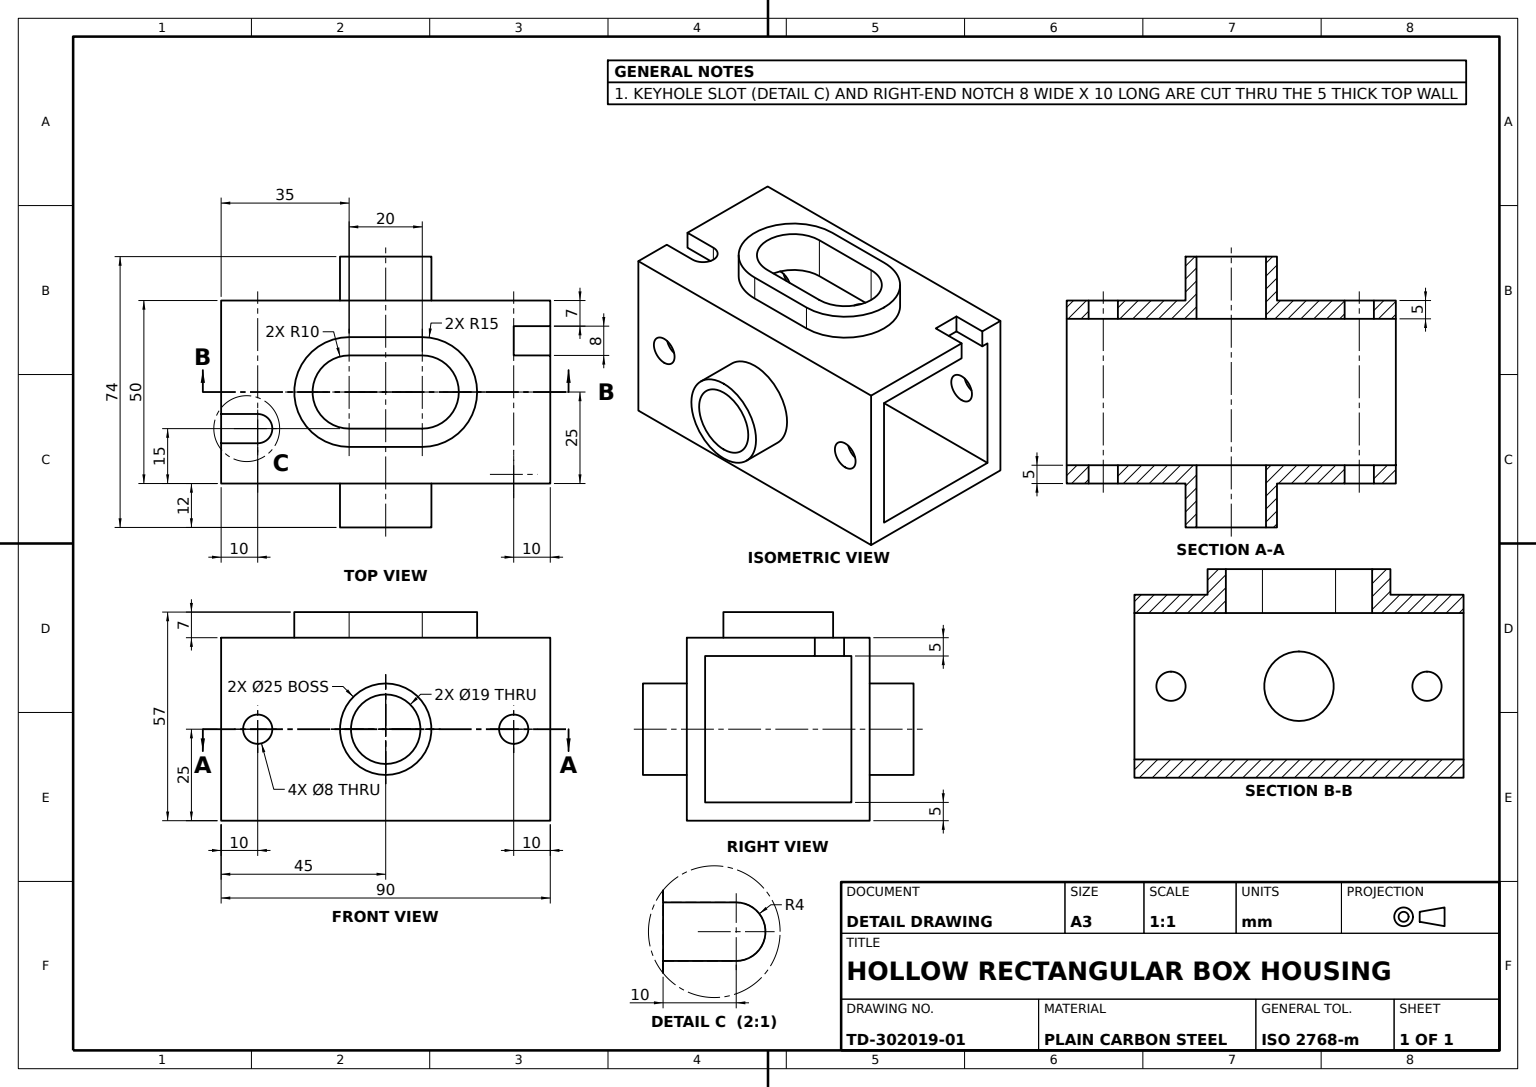
from build123d import *

# Parameters (mm, degrees)
TUBE_PROFILE_50X50X5_SKETCH_W   = 50
TUBE_PROFILE_50X50X5_SKETCH_H   = 50
TUBE_PROFILE_50X50X5_SKETCH_W_2 = 40
TUBE_PROFILE_50X50X5_SKETCH_H_2 = 40
SQUARE_TUBE_BODY_L90_DEPTH      = 90
KEYHOLE_NOTCH_SKETCH_W          = 8
KEYHOLE_NOTCH_SKETCH_H          = 10
KEYHOLE_NOTCHES_DEPTH           = 5
OBROUND_BOSS_DEPTH              = 7
OBROUND_START                   = -7
OBROUND_SLOT_CUT_DEPTH          = 7
SIDE_BOSS_AND_HOLES_SKETCH_R    = 12.5
SIDE_BOSS_AND_HOLES_SKETCH_R_2  = 9.5
SIDE_BOSS_25_DEPTH              = 12
SKETCH7_3_R                     = 4
SKETCH7_3_R_2                   = 9.5
SIDE_BORE_AND_HOLES_DEPTH       = 108.814655776


with BuildPart() as part:
    # Tube Profile 50x50x5 Sketch → Square Tube Body L90 (new body)
    with BuildSketch(Plane.XY):
        Rectangle(TUBE_PROFILE_50X50X5_SKETCH_W, TUBE_PROFILE_50X50X5_SKETCH_H)
        Rectangle(TUBE_PROFILE_50X50X5_SKETCH_W_2, TUBE_PROFILE_50X50X5_SKETCH_H_2, mode=Mode.SUBTRACT)
    extrude(amount=SQUARE_TUBE_BODY_L90_DEPTH)

    # Keyhole Notch Sketch → Keyhole Notches (cut)
    with BuildSketch(Plane(origin=(0, 25, 0), x_dir=(1, 0, 0), z_dir=(0, 1, 0))):
        with BuildLine():
            Line((14, -90), (14, -80))
            ThreePointArc((14, -80), (10, -76), (6, -80))
            Line((6, -80), (6, -90))
            Line((6, -90), (14, -90))
        make_face()
        with Locations((-14, -5)):
            Rectangle(KEYHOLE_NOTCH_SKETCH_W, KEYHOLE_NOTCH_SKETCH_H)
    extrude(amount=-KEYHOLE_NOTCHES_DEPTH, mode=Mode.SUBTRACT)

    # Obround Boss Sketch → Obround Boss (add)
    with BuildSketch(Plane(origin=(0, 25, 0), x_dir=(1, 0, 0), z_dir=(0, 1, 0))):
        with BuildLine():
            Line((15, -35), (15, -55))
            ThreePointArc((15, -55), (0, -70), (-15, -55))
            Line((-15, -55), (-15, -35))
            ThreePointArc((-15, -35), (0, -20), (15, -35))
        make_face()
        with BuildLine():
            Line((10, -35), (10, -55))
            ThreePointArc((10, -55), (0, -65), (-10, -55))
            Line((-10, -55), (-10, -35))
            ThreePointArc((-10, -35), (0, -25), (10, -35))
        make_face(mode=Mode.SUBTRACT)
    extrude(amount=OBROUND_BOSS_DEPTH)

    # Sketch6_2 → Obround Slot Cut (cut)
    with BuildSketch(Plane(origin=(0, 25, 0), x_dir=(1, 0, 0), z_dir=(0, 1, 0)).offset(OBROUND_START)):
        with BuildLine():
            Line((10, -35), (10, -55))
            ThreePointArc((10, -55), (0, -65), (-10, -55))
            Line((-10, -55), (-10, -35))
            ThreePointArc((-10, -35), (0, -25), (10, -35))
        make_face()
    extrude(amount=OBROUND_SLOT_CUT_DEPTH, mode=Mode.SUBTRACT)

    # Side Boss and Holes Sketch → Side Boss _25 (add)
    with BuildSketch(Plane(origin=(25, 0, 0), x_dir=(0, 0, -1), z_dir=(1, 0, 0))):
        with Locations(Location((-45, 0, 0), (0, 0, 270))):
            Circle(SIDE_BOSS_AND_HOLES_SKETCH_R)
        with Locations(Location((-45, 0, 0), (0, 0, 90))):
            Circle(SIDE_BOSS_AND_HOLES_SKETCH_R_2, mode=Mode.SUBTRACT)
    side_boss_25 = extrude(amount=SIDE_BOSS_25_DEPTH)

    # Sketch7_3 → Side Bore and Holes (cut, through all)
    with BuildSketch(Plane(origin=(25, 0, 0), x_dir=(0, 0, -1), z_dir=(1, 0, 0))):
        with Locations(Location((-80, 0, 0), (0, 0, 90))):
            Circle(SKETCH7_3_R)
        with Locations(Location((-10, 0, 0), (0, 0, 90))):
            Circle(SKETCH7_3_R)
        with Locations(Location((-45, 0, 0), (0, 0, 270))):
            Circle(SKETCH7_3_R_2)
    extrude(amount=-SIDE_BORE_AND_HOLES_DEPTH, mode=Mode.SUBTRACT)

    # Side Boss Mirror: Side Boss _25 across plane
    add(side_boss_25.mirror(Plane(origin=(0, 0, 0), x_dir=(0, 0, 1), z_dir=(1, 0, 0))))


solid = part.part
